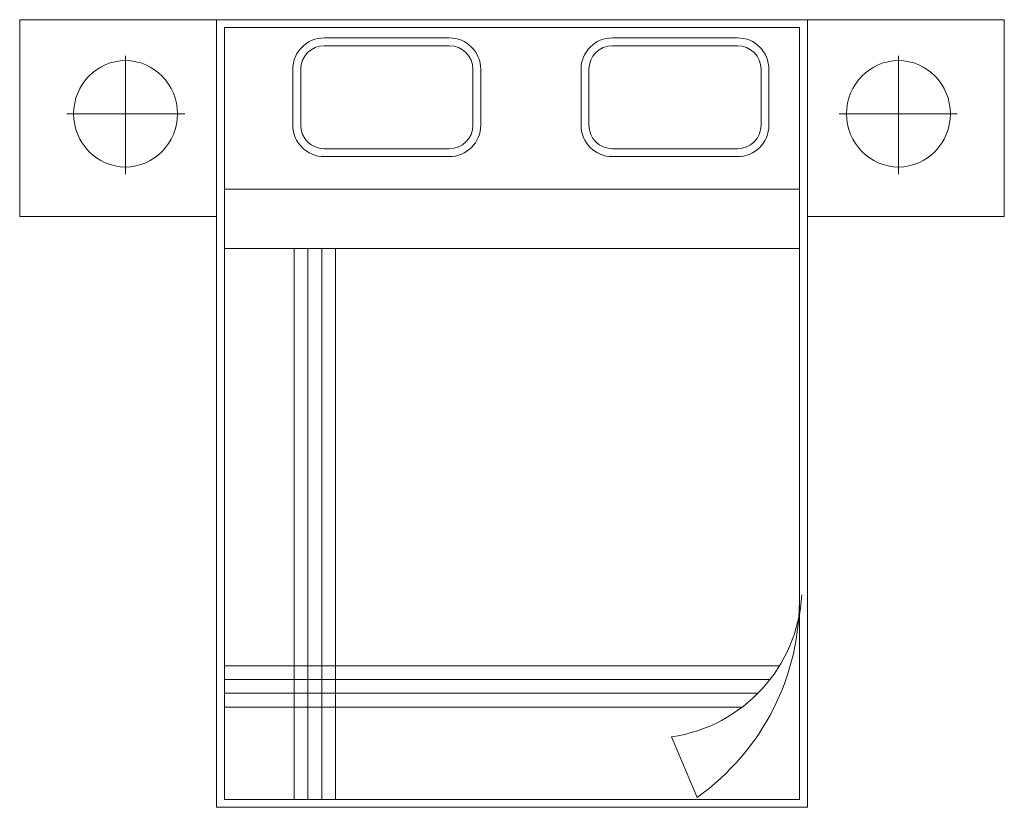
# Model space of a CAD drawing. Units: inches. Extents: x -20 to 10156, y 488 to 2970.
# Tile 6 of 6: x 7656 to 10156, y 970 to 2970. Entities that reach past the tile are written whole.
import ezdxf

# ---------------------------------------------------------------- set-up
doc = ezdxf.new("R2010")
doc.units = ezdxf.units.IN
doc.header["$MEASUREMENT"] = 0
doc.layers.add('A-FURN', color=8, linetype='Continuous', lineweight=18)

# ---------------------------------------------------------------- blocks, each defined once
blk = doc.blocks.new('A$C057D194F')
for p, q in [((0, 1.5, -0.1688), (0, 2, -0.1688)), ((0, 2, -0.1688), (0.5, 2, -0.1688)), ((0.5, 2, -0.1688), (0.5, 0, -0.1688)), ((2, 2, -0.1688), (0.5, 2, -0.1688)), ((1.98, 1.98, -0.1688), (0.52, 1.98, -0.1688)), ((0.52, 1.98, -0.1688), (0.52, 0.02, -0.1688)), ((1.98, 0.02, -0.1688), (1.98, 1.98, -0.1688)), ((2, 0, -0.1688), (2, 2, -0.1688)), ((2.5, 2, -0.1688), (2, 2, -0.1688)), ((2.5, 1.5, -0.1688), (2.5, 2, -0.1688)), ((1.0907, 1.9539, -0.1688), (0.7735, 1.9539, -0.1688)), ((1.8224, 1.9539, -0.1688), (1.5052, 1.9539, -0.1688)), ((1.0907, 1.9339, -0.1688), (0.7735, 1.9339, -0.1688)), ((1.8224, 1.9339, -0.1688), (1.5052, 1.9339, -0.1688)), ((0.2687, 1.9081, -0.1688), (0.2687, 1.761, -0.1688)), ((0.2687, 1.6081, -0.1688), (0.2687, 1.9081, -0.1688)), ((2.2313, 1.9081, -0.1688), (2.2313, 1.761, -0.1688)), ((2.2313, 1.6081, -0.1688), (2.2313, 1.9081, -0.1688)), ((0.6935, 1.8739, -0.1688), (0.6935, 1.7322, -0.1688)), ((0.7135, 1.8739, -0.1688), (0.7135, 1.7322, -0.1688)), ((1.1507, 1.7322, -0.1688), (1.1507, 1.8739, -0.1688)), ((1.1707, 1.7322, -0.1688), (1.1707, 1.8739, -0.1688)), ((1.4252, 1.8739, -0.1688), (1.4252, 1.7322, -0.1688)), ((1.4452, 1.8739, -0.1688), (1.4452, 1.7322, -0.1688)), ((1.8824, 1.7322, -0.1688), (1.8824, 1.8739, -0.1688)), ((1.9024, 1.7322, -0.1688), (1.9024, 1.8739, -0.1688)), ((0.4194, 1.761, -0.1688), (0.1194, 1.761, -0.1688)), ((0.2687, 1.761, -0.1688), (0.4194, 1.761, -0.1688)), ((0.2687, 1.761, -0.1688), (0.2687, 1.6081, -0.1688)), ((2.0806, 1.761, -0.1688), (2.3806, 1.761, -0.1688)), ((2.2313, 1.761, -0.1688), (2.0806, 1.761, -0.1688)), ((2.2313, 1.761, -0.1688), (2.2313, 1.6081, -0.1688)), ((0.7735, 1.6722, -0.1688), (1.0907, 1.6722, -0.1688)), ((0.7735, 1.6522, -0.1688), (1.0907, 1.6522, -0.1688)), ((1.5052, 1.6722, -0.1688), (1.8224, 1.6722, -0.1688)), ((1.5052, 1.6522, -0.1688), (1.8224, 1.6522, -0.1688)), ((1.98, 1.5693, -0.1688), (0.52, 1.5693, -0.1688)), ((0.5, 1.5, -0.1688), (0, 1.5, -0.1688)), ((2, 1.5, -0.1688), (2.5, 1.5, -0.1688)), ((1.98, 1.4193, -0.1688), (0.52, 1.4193, -0.1688)), ((0.6969, 0.02, -0.1688), (0.6969, 1.4193, -0.1688)), ((0.7319, 0.02, -0.1688), (0.7319, 1.4193, -0.1688)), ((0.7669, 0.02, -0.1688), (0.7669, 1.4193, -0.1688)), ((0.8019, 0.02, -0.1688), (0.8019, 1.4193, -0.1688)), ((0.52, 0.3595, -0.1688), (1.9292, 0.3595, -0.1688)), ((0.52, 0.3245, -0.1688), (1.905, 0.3245, -0.1688)), ((0.52, 0.2895, -0.1688), (1.8742, 0.2895, -0.1688)), ((0.52, 0.2545, -0.1688), (1.8344, 0.2545, -0.1688)), ((1.6548, 0.1789, -0.1688), (1.7198, 0.0251, -0.1688)), ((0.52, 0.02, -0.1688), (1.98, 0.02, -0.1688)), ((0.5, 0, -0.1688), (2, 0, -0.1688))]:
    blk.add_line(p, q)
for centre, radius, start, end in [((0.7735, 1.8739, -0.1688), 0.08, 90, 180), ((1.0907, 1.8739, -0.1688), 0.08, 0, 90), ((1.5052, 1.8739, -0.1688), 0.08, 90, 180), ((1.8224, 1.8739, -0.1688), 0.08, 0, 90), ((0.7735, 1.8739, -0.1688), 0.06, 90, 180), ((1.0907, 1.8739, -0.1688), 0.06, 0, 90), ((1.5052, 1.8739, -0.1688), 0.06, 90, 180), ((1.8224, 1.8739, -0.1688), 0.06, 0, 90), ((0.7735, 1.7322, -0.1688), 0.08, 180, 270), ((0.7735, 1.7322, -0.1688), 0.06, 180, 270), ((1.0907, 1.7322, -0.1688), 0.08, 270, 0), ((1.0907, 1.7322, -0.1688), 0.06, 270, 0), ((1.5052, 1.7322, -0.1688), 0.08, 180, 270), ((1.5052, 1.7322, -0.1688), 0.06, 180, 270), ((1.8224, 1.7322, -0.1688), 0.08, 270, 0), ((1.8224, 1.7322, -0.1688), 0.06, 270, 0), ((1.5992, 0.5623, -0.1688), 0.3874, 278.2518, 356.6808), ((1.363, 0.5286, -0.1688), 0.6171, 305.3295, 1.0459)]:
    blk.add_arc(centre, radius, start, end)
blk.add_ellipse((0.2687, 1.761, -0.1688), major_axis=(0, -0.1351), ratio=0.975448)
at = {"extrusion": (0, 0, -1)}
blk.add_ellipse((2.2313, 1.761, -0.1688), major_axis=(0, 0.1351), ratio=0.975448, dxfattribs=at)
for p in [(0.2687, 1.761, -0.1688), (2.2313, 1.761, -0.1688)]:
    blk.add_point(p)

msp = doc.modelspace()

# ---------------------------------------------------------------- block references
at = {"layer": 'A-FURN', "xscale": 1000, "yscale": 1000, "zscale": 1000}
msp.add_blockref('A$C057D194F', (7656.11, 969.51), dxfattribs=at)

doc.saveas('drawing.dxf')
